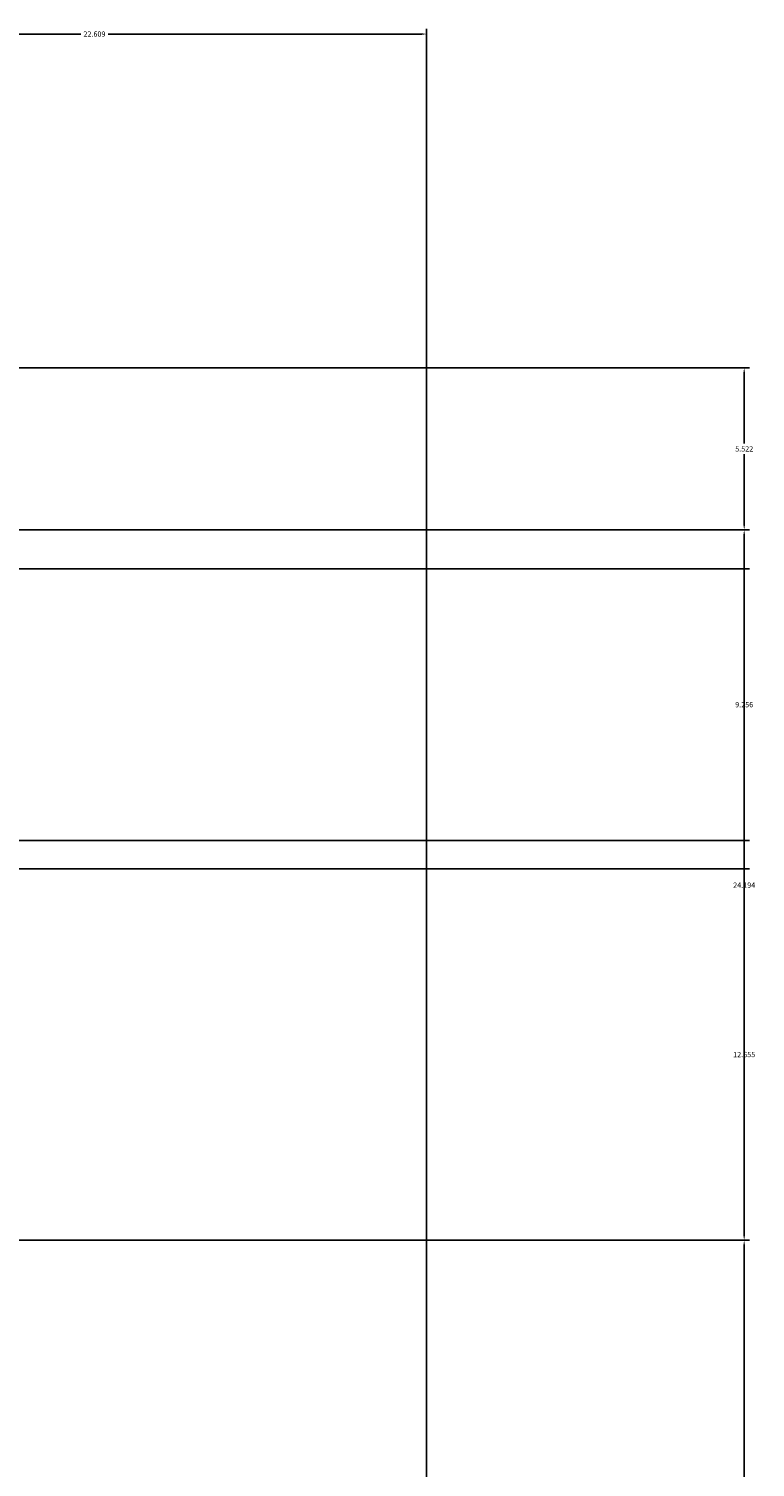
# Model space of a CAD drawing. Units: inches. Extents: x -117 to 121, y -77 to 40.
# Tile 45 of 45: x 96 to 121, y -10 to 39. Entities that reach past the tile are written whole.
import ezdxf

# ---------------------------------------------------------------- set-up
doc = ezdxf.new("R2010")
doc.units = ezdxf.units.IN
doc.header["$MEASUREMENT"] = 0
doc.layers.add('A-ANNO-DIMS', color=2, linetype='Continuous', lineweight=18)
doc.styles.get("Standard").update_dxf_attribs({"font": 'arial.ttf'})
doc.dimstyles.get("Standard").update_dxf_attribs({"dimtxt": 0.18, "dimasz": 0.18, "dimexe": 0.18, "dimexo": 0.0625, "dimgap": 0.09, "dimtad": 0, "dimtih": 1, "dimtoh": 1, "dimdec": 4, "dimzin": 0, "dimdsep": 46, "dimtxsty": 'Standard', "dimcen": 0.09, "dimadec": 0, "dimazin": 0, "dimtfac": 1, "dimtdec": 4, "dimtofl": 0, "dimtmove": 0, "dimatfit": 3, "dimfxl": 1, "dimtolj": 1, "dimtzin": 0, "dimarcsym": 0})

# ---------------------------------------------------------------- blocks, each defined once
blk = doc.blocks.new('*D15')
at = {"layer": 'A-ANNO-DIMS', "color": 0, "lineweight": -2, "transparency": 16777216}
for p, q in [((87.304, -2.653), (120.84, -2.653)), ((120.66, -2.833), (120.66, -20.595)), ((120.66, -38.722), (120.66, -20.959)), ((90.611, -38.902), (120.84, -38.902))]:
    blk.add_line(p, q, dxfattribs=at)
at = {"layer": 'A-ANNO-DIMS', "color": 0, "transparency": 16777216}
for points in [[(120.63, -2.833), (120.69, -2.833), (120.66, -2.653)], [(120.63, -38.722), (120.69, -38.722), (120.66, -38.902)]]:
    blk.add_solid(points, dxfattribs=at)
at = {"layer": 'Defpoints', "color": 0, "transparency": 16777216}
for p in [(87.242, -2.653), (90.549, -38.902), (120.66, -38.902)]:
    blk.add_point(p, dxfattribs=at)
at = {"layer": 'A-ANNO-DIMS', "color": 0, "transparency": 16777216, "insert": (120.66, -20.777), "char_height": 0.18, "attachment_point": 5}
blk.add_mtext('\\A1;36.25', dxfattribs=at)
blk = doc.blocks.new('*D16')
at = {"layer": 'A-ANNO-DIMS', "color": 0, "lineweight": -2, "transparency": 16777216}
for p, q in [((70.862, 21.541), (120.84, 21.541)), ((120.66, 21.361), (120.66, 9.626)), ((120.66, -2.473), (120.66, 9.262)), ((87.304, -2.653), (120.84, -2.653))]:
    blk.add_line(p, q, dxfattribs=at)
at = {"layer": 'A-ANNO-DIMS', "color": 0, "transparency": 16777216}
for points in [[(120.63, 21.361), (120.69, 21.361), (120.66, 21.541)], [(120.63, -2.473), (120.69, -2.473), (120.66, -2.653)]]:
    blk.add_solid(points, dxfattribs=at)
at = {"layer": 'Defpoints', "color": 0, "transparency": 16777216}
for p in [(70.8, 21.541), (87.242, -2.653), (120.66, -2.653)]:
    blk.add_point(p, dxfattribs=at)
at = {"layer": 'A-ANNO-DIMS', "color": 0, "transparency": 16777216, "insert": (120.66, 9.444), "char_height": 0.18, "attachment_point": 5}
blk.add_mtext('\\A1;24.194', dxfattribs=at)
blk = doc.blocks.new('*D17')
at = {"layer": 'A-ANNO-DIMS', "color": 0, "lineweight": -2, "transparency": 16777216}
for p, q in [((14.041, 27.063), (120.84, 27.063)), ((120.66, 26.883), (120.66, 24.484)), ((120.66, 21.721), (120.66, 24.12)), ((70.862, 21.541), (120.84, 21.541))]:
    blk.add_line(p, q, dxfattribs=at)
at = {"layer": 'A-ANNO-DIMS', "color": 0, "transparency": 16777216}
for points in [[(120.63, 26.883), (120.69, 26.883), (120.66, 27.063)], [(120.63, 21.721), (120.69, 21.721), (120.66, 21.541)]]:
    blk.add_solid(points, dxfattribs=at)
at = {"layer": 'Defpoints', "color": 0, "transparency": 16777216}
for p in [(13.978, 27.063), (70.8, 21.541), (120.66, 21.541)]:
    blk.add_point(p, dxfattribs=at)
at = {"layer": 'A-ANNO-DIMS', "color": 0, "transparency": 16777216, "insert": (120.66, 24.302), "char_height": 0.18, "attachment_point": 5}
blk.add_mtext('\\A1;5.522', dxfattribs=at)
blk = doc.blocks.new('*D24')
at = {"layer": 'A-ANNO-DIMS', "color": 0, "lineweight": -2, "transparency": 16777216}
for p, q in [((87.242, 3.166), (87.242, 38.61)), ((87.422, 38.43), (98.081, 38.43)), ((109.67, 38.43), (99.011, 38.43)), ((109.85, -61.313), (109.85, 38.61))]:
    blk.add_line(p, q, dxfattribs=at)
at = {"layer": 'A-ANNO-DIMS', "color": 0, "transparency": 16777216}
for points in [[(87.422, 38.46), (87.422, 38.4), (87.242, 38.43)], [(109.67, 38.46), (109.67, 38.4), (109.85, 38.43)]]:
    blk.add_solid(points, dxfattribs=at)
at = {"layer": 'Defpoints', "color": 0, "transparency": 16777216}
for p in [(109.85, 38.43), (87.242, 3.104), (109.85, -61.376)]:
    blk.add_point(p, dxfattribs=at)
at = {"layer": 'A-ANNO-DIMS', "color": 0, "transparency": 16777216, "insert": (98.546, 38.43), "char_height": 0.18, "attachment_point": 5}
blk.add_mtext('\\A1;22.609', dxfattribs=at)
blk = doc.blocks.new('*D54')
at = {"layer": 'A-ANNO-DIMS', "color": 0, "lineweight": -2, "transparency": 16777216}
for p, q in [((51.654, 20.218), (120.84, 20.218)), ((120.66, 20.038), (120.66, 15.772)), ((120.66, 11.142), (120.66, 15.408)), ((51.753, 10.962), (120.84, 10.962))]:
    blk.add_line(p, q, dxfattribs=at)
at = {"layer": 'A-ANNO-DIMS', "color": 0, "transparency": 16777216}
for points in [[(120.63, 20.038), (120.69, 20.038), (120.66, 20.218)], [(120.63, 11.142), (120.69, 11.142), (120.66, 10.962)]]:
    blk.add_solid(points, dxfattribs=at)
at = {"layer": 'Defpoints', "color": 0, "transparency": 16777216}
for p in [(51.591, 20.218), (120.66, 20.218), (51.69, 10.962)]:
    blk.add_point(p, dxfattribs=at)
at = {"layer": 'A-ANNO-DIMS', "color": 0, "transparency": 16777216, "insert": (120.66, 15.59), "char_height": 0.18, "attachment_point": 5}
blk.add_mtext('\\A1;9.256', dxfattribs=at)
blk = doc.blocks.new('*D55')
at = {"layer": 'A-ANNO-DIMS', "color": 0, "lineweight": -2, "transparency": 16777216}
for p, q in [((65.473, 10.002), (120.84, 10.002)), ((120.66, 9.822), (120.66, 3.857)), ((120.66, -2.473), (120.66, 3.493)), ((65.624, -2.653), (120.84, -2.653))]:
    blk.add_line(p, q, dxfattribs=at)
at = {"layer": 'A-ANNO-DIMS', "color": 0, "transparency": 16777216}
for points in [[(120.63, 9.822), (120.69, 9.822), (120.66, 10.002)], [(120.63, -2.473), (120.69, -2.473), (120.66, -2.653)]]:
    blk.add_solid(points, dxfattribs=at)
at = {"layer": 'Defpoints', "color": 0, "transparency": 16777216}
for p in [(65.411, 10.002), (120.66, 10.002), (65.562, -2.653)]:
    blk.add_point(p, dxfattribs=at)
at = {"layer": 'A-ANNO-DIMS', "color": 0, "transparency": 16777216, "insert": (120.66, 3.675), "char_height": 0.18, "attachment_point": 5}
blk.add_mtext('\\A1;12.655', dxfattribs=at)

msp = doc.modelspace()

# ---------------------------------------------------------------- dimensions: what is measured, and where the dimension line sits
at = {"layer": 'A-ANNO-DIMS'}
dim = msp.add_linear_dim(base=(109.8502, 38.4297), p1=(87.2416, 3.1036), p2=(109.8502, -61.3756), dimstyle='Standard', override={"dimdec": 3, "dimlfac": 1, "dimrnd": 0, "dimzin": 0, "dimdsep": 46, "dimlunit": 2}, dxfattribs=at)
dim.commit()
dim.dimension.update_dxf_attribs({"geometry": '*D24', "text_midpoint": (98.5459, 38.4297)})
for base, p1, p2, override, picture, middle in [((120.6602, 21.5414), (13.9784, 27.0634), (70.8, 21.5414), {"dimdec": 3, "dimlfac": 1, "dimrnd": 0, "dimzin": 0, "dimdsep": 46, "dimlunit": 2}, '*D17', (120.6602, 24.3024)), ((120.6602, -2.6528), (70.8, 21.5414), (87.2416, -2.6528), {"dimdec": 3, "dimlfac": 1, "dimrnd": 0, "dimzin": 0, "dimdsep": 46, "dimlunit": 2}, '*D16', (120.6602, 9.4443)), ((120.6602, 20.2181), (51.6901, 10.9623), (51.5915, 20.2181), {"dimdec": 3, "dimlfac": 1, "dimrnd": 0, "dimzin": 0, "dimdsep": 46, "dimlunit": 2}, '*D54', (120.6602, 15.5902)), ((120.6602, 10.0025), (65.562, -2.6528), (65.4109, 10.0025), {"dimdec": 3, "dimlfac": 1, "dimrnd": 0, "dimzin": 0, "dimdsep": 46, "dimlunit": 2}, '*D55', (120.6602, 3.6749)), ((120.6602, -38.9022), (87.2416, -2.6528), (90.5486, -38.9022), {"dimdec": 2, "dimlfac": 1, "dimrnd": 0, "dimzin": 0, "dimdsep": 46, "dimlunit": 2}, '*D15', (120.6602, -20.7775))]:
    dim = msp.add_linear_dim(base=base, p1=p1, p2=p2, angle=90, dimstyle='Standard', override=override, dxfattribs=at)
    dim.commit()
    dim.dimension.update_dxf_attribs({"geometry": picture, "text_midpoint": middle})

doc.saveas('drawing.dxf')
